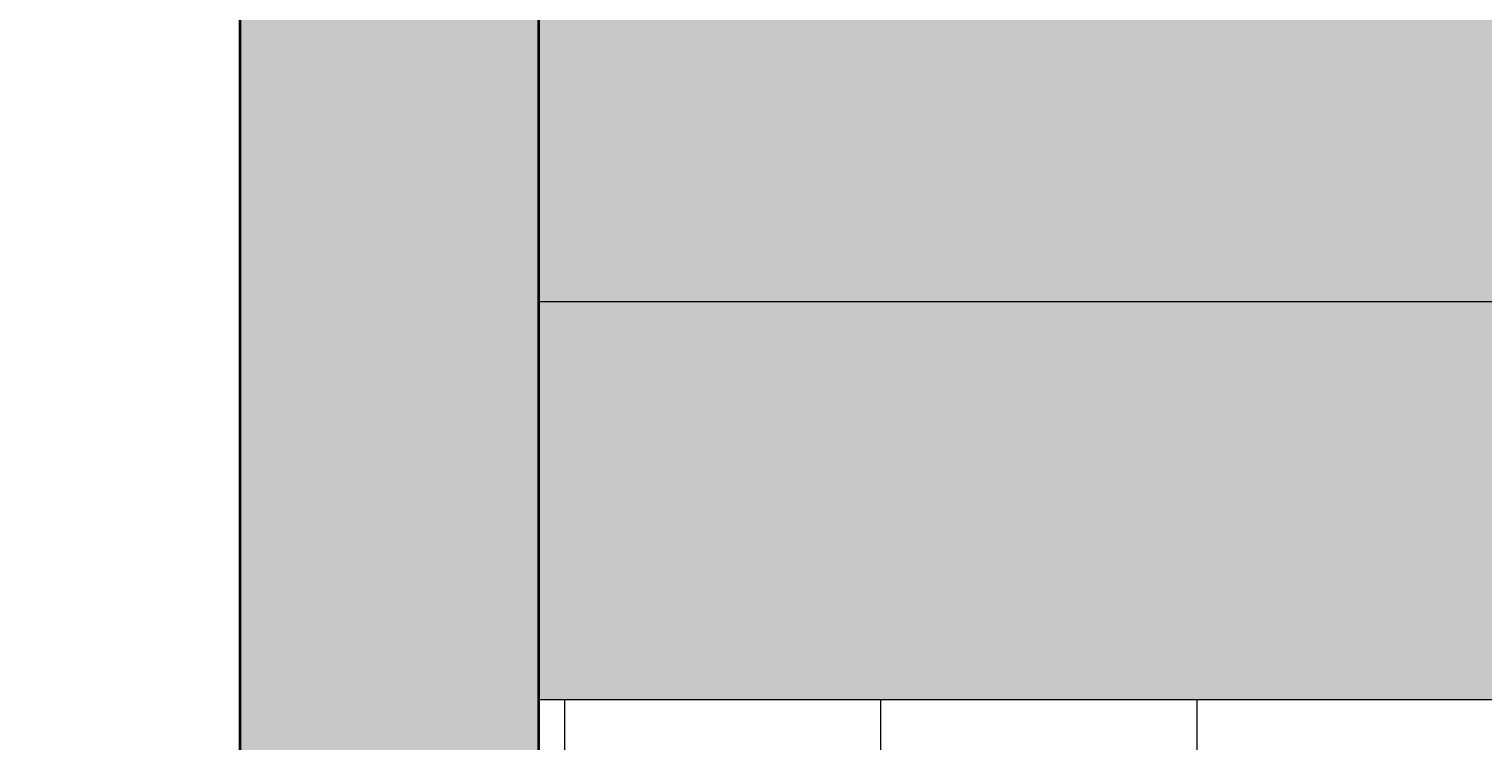
# Model space of a CAD drawing. Units: inches. Extents: x 84 to 1044, y -280 to 906.
# Tile 68 of 105: x 689 to 733, y 387 to 408. Entities that reach past the tile are written whole.
import ezdxf

# ---------------------------------------------------------------- set-up
doc = ezdxf.new("R2010")
doc.units = ezdxf.units.IN
for name, color, linetype, lineweight in [('A-ANNO-DIMS', 2, 'Continuous', 18), ('A-STAIRCASE', 144, 'Continuous', 18), ('WALL', 250, 'Continuous', 35)]:
    doc.layers.add(name, color=color, linetype=linetype, lineweight=lineweight)
for name, color, linetype, lineweight, true_color in [('A-FLOR-PATT', 251, 'Continuous', 9, 0x705861), ('A-FLOR-STRS-PATT', 35, 'Continuous', 9, 0x947764), ('A-WALL-PATT', 251, 'Continuous', 9, 0x636466), ('L-PLNT-PATT', 9, 'Continuous', 9, 0xafd9aa)]:
    doc.layers.add(name, color=color, linetype=linetype, lineweight=lineweight, true_color=true_color)
doc.styles.get("Standard").update_dxf_attribs({"font": 'arial.ttf'})
doc.dimstyles.get("Standard").update_dxf_attribs({"dimtxt": 0.18, "dimasz": 0.18, "dimexe": 0.18, "dimexo": 0.0625, "dimgap": 0.09, "dimtad": 0, "dimtih": 1, "dimtoh": 1, "dimdec": 4, "dimzin": 0, "dimdsep": 46, "dimtxsty": 'Standard', "dimcen": 0.09, "dimadec": 0, "dimazin": 0, "dimtfac": 1, "dimtdec": 4, "dimtofl": 0, "dimtmove": 0, "dimatfit": 3, "dimfxl": 1, "dimtolj": 1, "dimtzin": 0, "dimarcsym": 0})

# ---------------------------------------------------------------- blocks, each defined once
blk = doc.blocks.new('*D62')
at = {"layer": 'A-ANNO-DIMS', "color": 0, "lineweight": -2, "transparency": 16777216}
for p, q in [((203.179, 709.183), (203.179, 905.9)), ((896.074, 400.183), (896.074, 905.9)), ((203.359, 905.72), (549.232, 905.72)), ((895.894, 905.72), (550.021, 905.72))]:
    blk.add_line(p, q, dxfattribs=at)
at = {"layer": 'A-ANNO-DIMS', "color": 0, "transparency": 16777216}
for points in [[(203.359, 905.75), (203.359, 905.69), (203.179, 905.72)], [(895.894, 905.75), (895.894, 905.69), (896.074, 905.72)]]:
    blk.add_solid(points, dxfattribs=at)
at = {"layer": 'Defpoints', "color": 0, "transparency": 16777216}
for p in [(896.074, 905.72), (203.179, 709.12), (896.074, 400.12)]:
    blk.add_point(p, dxfattribs=at)
at = {"layer": 'A-ANNO-DIMS', "color": 0, "transparency": 16777216, "insert": (549.627, 905.72), "char_height": 0.18, "attachment_point": 5}
blk.add_mtext('\\A1;692.9', dxfattribs=at)

msp = doc.modelspace()

# ---------------------------------------------------------------- hatches: boundary and pattern name
at = {"layer": 'A-FLOR-PATT', "transparency": 33554597}
h = msp.add_hatch(dxfattribs=at)
h.set_pattern_fill('ANSI37', color=256, scale=3, angle=45)
h.paths.add_polyline_path([(833.074, 388.12), (704.074, 388.12), (704.074, 370.12), (695.074, 370.12), (695.074, 334.12), (732.574, 334.12), (804.574, 334.12), (833.074, 334.12), (833.074, 364.12)])
at = {"layer": 'A-FLOR-STRS-PATT', "transparency": 33554567}
h = msp.add_hatch(color=256, dxfattribs=at)
h.dxf.hatch_style = 1
h.paths.add_polyline_path([(833.074, 400.12), (704.074, 400.12), (704.074, 388.12), (833.074, 388.12)])
at = {"layer": 'A-WALL-PATT', "transparency": 33554597}
h = msp.add_hatch(color=256, dxfattribs=at)
h.dxf.hatch_style = 1
h.paths.add_polyline_path([(671.074, 100.12), (647.074, 100.12), (647.074, 160.12), (641.074, 160.12), (620.824, 160.12), (620.824, 151.12), (638.074, 151.12), (638.074, 91.12), (671.074, 91.12)])
h.paths.add_polyline_path([(791.074, 100.12), (743.074, 100.12), (743.074, 91.12), (791.074, 91.12)])
h.paths.add_polyline_path([(896.074, 346.12), (887.074, 346.12), (887.074, 334.12), (870.955, 334.12), (833.074, 334.12), (804.574, 334.12), (804.574, 328.12), (887.074, 328.12), (887.074, 100.12), (863.074, 100.12), (863.074, 91.12), (896.074, 91.12)])
h.paths.add_polyline_path([(507.574, 154.729), (507.574, 160.12), (464.074, 160.12), (464.074, 247.12), (641.074, 247.12), (641.074, 208.12), (647.074, 208.12), (647.074, 328.12), (659.074, 328.12), (659.074, 334.12), (617.074, 334.12), (617.074, 328.12), (641.074, 328.12), (641.074, 256.12), (545.074, 256.12), (545.074, 328.12), (569.074, 328.12), (569.074, 334.12), (518.074, 334.12), (518.074, 325.12), (536.074, 325.12), (536.074, 256.12), (464.074, 256.12), (464.074, 325.12), (482.074, 325.12), (482.074, 334.12), (455.074, 334.12), (455.074, 160.12), (413.127, 160.12), (413.127, 151.12), (455.074, 151.12), (455.074, 91.12), (464.074, 91.12), (464.074, 151.12), (507.574, 151.12)])
h.paths.add_polyline_path([(572.824, 160.12), (555.574, 160.12), (555.574, 151.12), (572.824, 151.12)], flags=17)
h.paths.add_polyline_path([(341.127, 160.12), (299.179, 160.12), (299.179, 211.12), (294.179, 211.12), (290.179, 211.12), (290.179, 151.12), (341.127, 151.12)])
h.paths.add_polyline_path([(299.179, 256.12), (212.179, 256.12), (212.179, 274.12), (203.179, 274.12), (203.179, 247.12), (299.179, 247.12)])
h.paths.add_polyline_path([(212.179, 514.12), (398.074, 514.12), (398.074, 519.12), (398.074, 520.12), (212.179, 520.12), (212.179, 574.12), (203.179, 574.12), (203.179, 310.12), (212.179, 310.12), (212.179, 328.12), (290.179, 328.12), (290.179, 292.12), (299.179, 292.12), (299.179, 328.12), (332.179, 328.12), (332.179, 334.12), (212.179, 334.12)])
h.paths.add_polyline_path([(287.127, 709.12), (203.179, 709.12), (203.179, 646.12), (212.179, 646.12), (212.179, 700.12), (287.127, 700.12)])
h.paths.add_polyline_path([(470.074, 709.12), (359.127, 709.12), (359.127, 700.12), (434.074, 700.12), (434.074, 574.12), (440.074, 574.12), (440.074, 622.12), (464.074, 622.12), (464.074, 628.12), (440.074, 628.12), (440.074, 700.12), (470.074, 700.12)])
h.paths.add_polyline_path([(572.074, 709.12), (506.074, 709.12), (506.074, 700.12), (536.074, 700.12), (536.074, 628.12), (494.074, 628.12), (494.074, 622.12), (536.074, 622.12), (536.074, 520.12), (440.074, 520.12), (440.074, 544.12), (434.074, 544.12), (434.074, 514.12), (644.074, 514.12), (644.074, 519.12), (644.074, 544.12), (638.074, 544.12), (638.074, 520.12), (542.074, 520.12), (542.074, 622.12), (584.074, 622.12), (584.074, 628.12), (542.074, 628.12), (542.074, 700.12), (572.074, 700.12)])
h.paths.add_polyline_path([(698.074, 709.12), (608.074, 709.12), (608.074, 700.12), (638.074, 700.12), (638.074, 628.12), (614.074, 628.12), (614.074, 622.12), (638.074, 622.12), (638.074, 574.12), (644.074, 574.12), (644.074, 700.12), (698.074, 700.12)])
h.paths.add_polyline_path([(833.074, 709.12), (770.074, 709.12), (770.074, 700.12), (824.074, 700.12), (824.074, 646.12), (833.074, 646.12)])
h.paths.add_polyline_path([(833.074, 574.12), (824.074, 574.12), (824.074, 520.12), (791.244, 520.12), (712.904, 520.12), (680.074, 520.12), (680.074, 514.12), (695.074, 514.12), (695.074, 491.62), (704.074, 491.62), (704.074, 511.12), (833.074, 511.12)])
h.paths.add_polyline_path([(704.074, 419.62), (695.074, 419.62), (695.074, 370.12), (704.074, 370.12)])
h.paths.add_polyline_path([(896.074, 400.12), (833.074, 400.12), (833.074, 364.12), (839.074, 364.12), (839.074, 394.12), (887.074, 394.12), (887.074, 382.12), (896.074, 382.12)])
h.paths.add_polyline_path([(732.574, 334.12), (695.074, 334.12), (695.074, 328.12), (732.574, 328.12)])
at = {"layer": 'L-PLNT-PATT', "transparency": 33554597}
h = msp.add_hatch(color=256, dxfattribs=at)
h.dxf.hatch_style = 1
h.paths.add_polyline_path([(896.074, 511.12), (704.074, 511.12), (704.074, 491.62), (704.074, 419.62), (704.074, 400.12), (833.074, 400.12), (896.074, 400.12)])

# ---------------------------------------------------------------- linework, layer by layer
at = {"layer": 'A-STAIRCASE'}
for p, q in [((833.074, 400.12), (704.074, 400.12)), ((833.074, 388.12), (704.074, 388.12))]:
    msp.add_line(p, q, dxfattribs=at)
at = {"layer": 'WALL'}
for p, q in [((695.074, 370.12), (695.074, 419.62)), ((704.074, 370.12), (704.074, 419.62))]:
    msp.add_line(p, q, dxfattribs=at)

# ---------------------------------------------------------------- dimensions: what is measured, and where the dimension line sits
at = {"layer": 'A-ANNO-DIMS'}
dim = msp.add_linear_dim(base=(896.074, 905.72), p1=(203.179, 709.12), p2=(896.074, 400.12), dimstyle='Standard', override={"dimdec": 1, "dimlfac": 1, "dimrnd": 0, "dimzin": 0, "dimdsep": 46, "dimlunit": 2}, dxfattribs=at)
dim.commit()
dim.dimension.update_dxf_attribs({"geometry": '*D62', "text_midpoint": (549.627, 905.72)})

doc.saveas('drawing.dxf')
